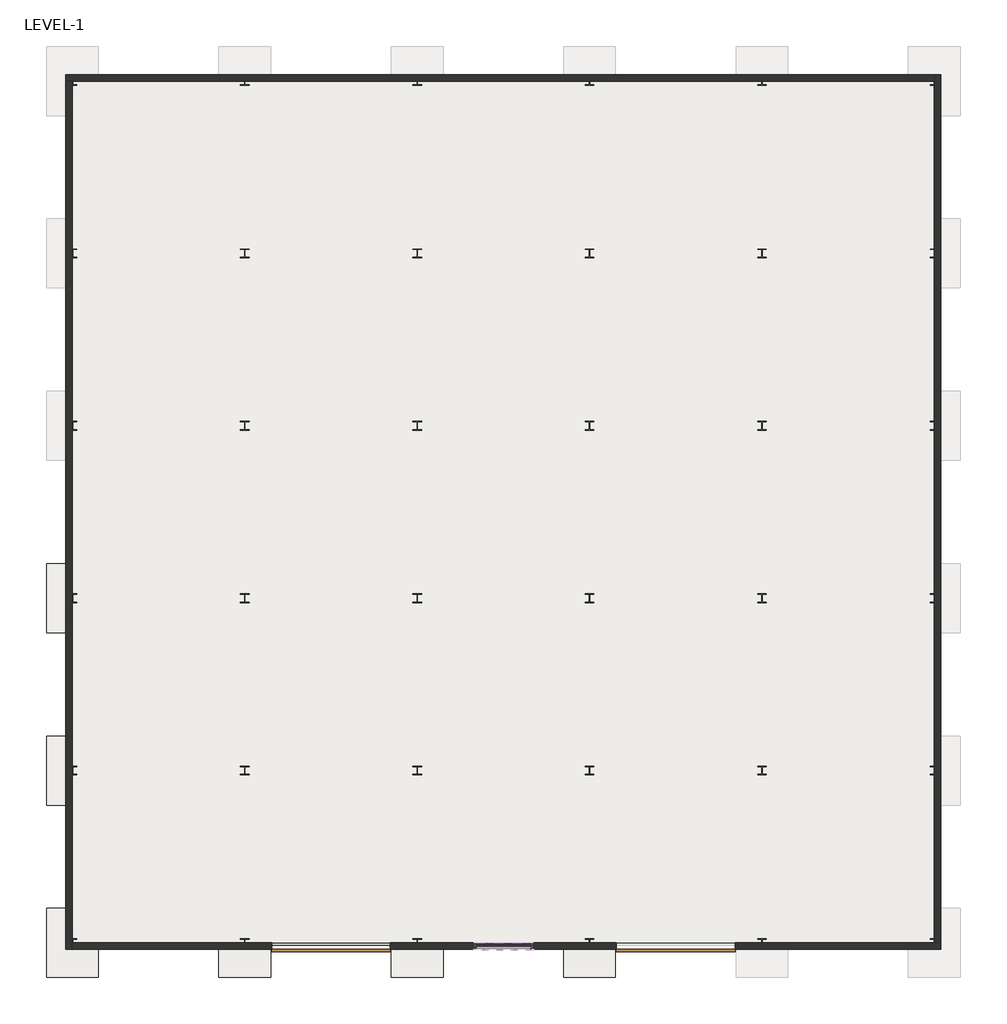
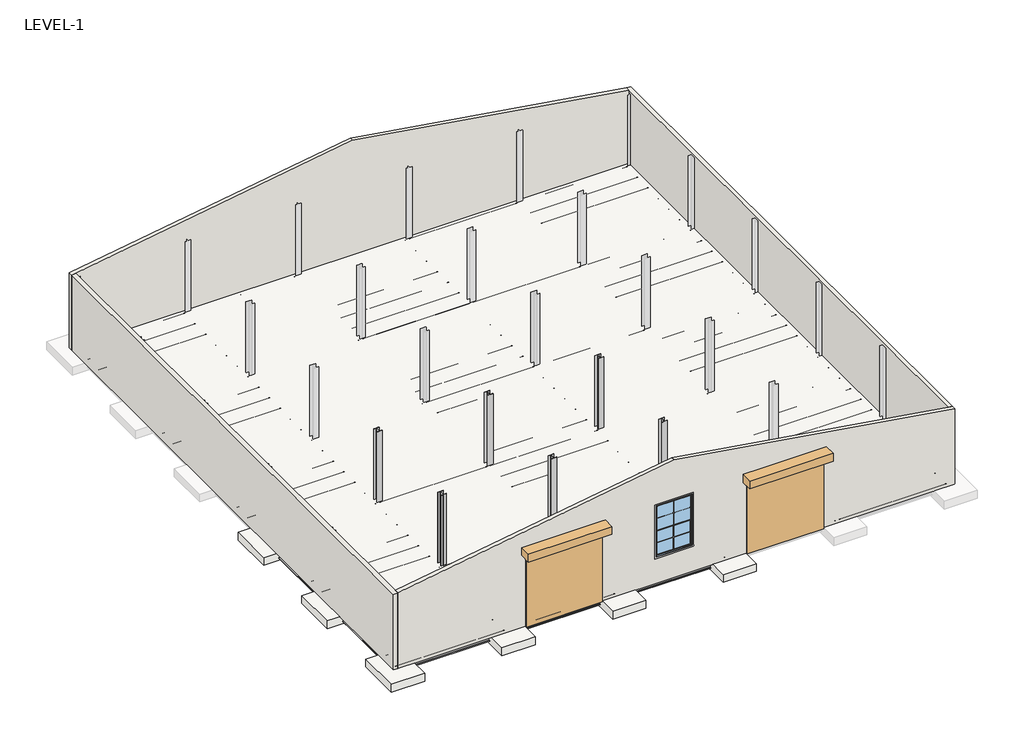
# One storey, part 1 of 3: 51 beams, 13 slabs, 12 columns, 4 walls, 2 doors, 1 window.
"""IFC4 building model written with IfcOpenShell, lengths in millimetres."""

from ifc_helpers import new_model, si_unit, frame, origin, place, context, project, spatial, polyline, outline, extrude, faceted_brep, transform, mapped, element, save
from components import ub_universal_beams_ub305x165x40_15f88fa9, ub_universal_beams_ub305x165x40_f918ae41, ub_universal_beams_ub305x165x40_f15b2736, ub_universal_beams_ub305x165x40_694d595e, uc_universal_columns_column_uc305x305x97_11a20181, m_door_overhead_rolling_4200_x_4200mm_2c196bb8, m_door_overhead_rolling_4200_x_4200mm_f21f583b, slab_7b69f09a, m_window_double_hung_2000_x_3000mm_b5dbafc5

model = new_model("IFC4")

# Units and contexts
model_context = context("Model", 3, world=origin())
ifc_project = project(units=[si_unit("LENGTHUNIT", "METRE", prefix="MILLI")], contexts=[model_context])

# Site, building, storey
site = spatial("IfcSite", under=ifc_project)
building = spatial("IfcBuilding", under=site)
storey = spatial("IfcBuildingStorey", under=building, Name="LEVEL-1", Elevation=0.0)

# Beams
placement = place(None, origin())
ub_universal_beams_ub305x165x40_shape = ub_universal_beams_ub305x165x40_15f88fa9(model_context)
element("IfcBeam", 1, ObjectType="UB-Universal Beams : UB305x165x40", at=placement, inside=storey, context=model_context, shape_type="MappedRepresentation", body=[
    mapped(ub_universal_beams_ub305x165x40_shape, transform((-15492.3332854, -104.4765895, -151.7), x_axis=(1.0, 0.0, 0.0), y_axis=(0.0, 1.0, 0.0), z_axis=(0.0, 0.0, 1.0))),
])
element("IfcBeam", 2, ObjectType="UB-Universal Beams : UB305x165x40", at=placement, inside=storey, context=model_context, shape_type="MappedRepresentation", body=[
    mapped(ub_universal_beams_ub305x165x40_shape, transform((-15492.3332854, -1120.4765895, -151.7), x_axis=(1.0, 0.0, 0.0), y_axis=(0.0, 1.0, 0.0), z_axis=(0.0, 0.0, 1.0))),
])
element("IfcBeam", 3, ObjectType="UB-Universal Beams : UB305x165x40", at=placement, inside=storey, context=model_context, shape_type="MappedRepresentation", body=[
    mapped(ub_universal_beams_ub305x165x40_shape, transform((-15492.3332854, -3152.4765895, -151.7), x_axis=(1.0, 0.0, 0.0), y_axis=(0.0, 1.0, 0.0), z_axis=(0.0, 0.0, 1.0))),
])
element("IfcBeam", 4, ObjectType="UB-Universal Beams : UB305x165x40", at=placement, inside=storey, context=model_context, shape_type="MappedRepresentation", body=[
    mapped(ub_universal_beams_ub305x165x40_shape, transform((-15492.3332854, -4168.4765895, -151.7), x_axis=(1.0, 0.0, 0.0), y_axis=(0.0, 1.0, 0.0), z_axis=(0.0, 0.0, 1.0))),
])
element("IfcBeam", 5, ObjectType="UB-Universal Beams : UB305x165x40", at=placement, inside=storey, context=model_context, shape_type="MappedRepresentation", body=[
    mapped(ub_universal_beams_ub305x165x40_shape, transform((-15492.3332854, -5184.4765895, -151.7), x_axis=(1.0, 0.0, 0.0), y_axis=(0.0, 1.0, 0.0), z_axis=(0.0, 0.0, 1.0))),
])
element("IfcBeam", 6, ObjectType="UB-Universal Beams : UB305x165x40", at=placement, inside=storey, context=model_context, shape_type="MappedRepresentation", body=[
    mapped(ub_universal_beams_ub305x165x40_shape, transform((-15492.3332854, -6200.4765895, -151.7), x_axis=(1.0, 0.0, 0.0), y_axis=(0.0, 1.0, 0.0), z_axis=(0.0, 0.0, 1.0))),
])
element("IfcBeam", 7, ObjectType="UB-Universal Beams : UB305x165x40", at=placement, inside=storey, context=model_context, shape_type="MappedRepresentation", body=[
    mapped(ub_universal_beams_ub305x165x40_shape, transform((-15492.3332854, -7216.4765895, -151.7), x_axis=(1.0, 0.0, 0.0), y_axis=(0.0, 1.0, 0.0), z_axis=(0.0, 0.0, 1.0))),
])
element("IfcBeam", 8, ObjectType="UB-Universal Beams : UB305x165x40", at=placement, inside=storey, context=model_context, shape_type="MappedRepresentation", body=[
    mapped(ub_universal_beams_ub305x165x40_shape, transform((-15492.3332854, -9248.4765895, -151.7), x_axis=(1.0, 0.0, 0.0), y_axis=(0.0, 1.0, 0.0), z_axis=(0.0, 0.0, 1.0))),
])
element("IfcBeam", 9, ObjectType="UB-Universal Beams : UB305x165x40", at=placement, inside=storey, context=model_context, shape_type="MappedRepresentation", body=[
    mapped(ub_universal_beams_ub305x165x40_shape, transform((-15492.3332854, -10264.4765895, -151.7), x_axis=(1.0, 0.0, 0.0), y_axis=(0.0, 1.0, 0.0), z_axis=(0.0, 0.0, 1.0))),
])
element("IfcBeam", 10, ObjectType="UB-Universal Beams : UB305x165x40", at=placement, inside=storey, context=model_context, shape_type="MappedRepresentation", body=[
    mapped(ub_universal_beams_ub305x165x40_shape, transform((-15492.3332854, -11280.4765895, -151.7), x_axis=(1.0, 0.0, 0.0), y_axis=(0.0, 1.0, 0.0), z_axis=(0.0, 0.0, 1.0))),
])
element("IfcBeam", 11, ObjectType="UB-Universal Beams : UB305x165x40", at=placement, inside=storey, context=model_context, shape_type="MappedRepresentation", body=[
    mapped(ub_universal_beams_ub305x165x40_shape, transform((-15492.3332854, -12296.4765895, -151.7), x_axis=(1.0, 0.0, 0.0), y_axis=(0.0, 1.0, 0.0), z_axis=(0.0, 0.0, 1.0))),
])
element("IfcBeam", 12, ObjectType="UB-Universal Beams : UB305x165x40", at=placement, inside=storey, context=model_context, shape_type="MappedRepresentation", body=[
    mapped(ub_universal_beams_ub305x165x40_shape, transform((-15492.3332854, -13312.4765895, -151.7), x_axis=(1.0, 0.0, 0.0), y_axis=(0.0, 1.0, 0.0), z_axis=(0.0, 0.0, 1.0))),
])
element("IfcBeam", 13, ObjectType="UB-Universal Beams : UB305x165x40", at=placement, inside=storey, context=model_context, shape_type="MappedRepresentation", body=[
    mapped(ub_universal_beams_ub305x165x40_shape, transform((-3300.3332854, -104.4765895, -151.7), x_axis=(1.0, 0.0, 0.0), y_axis=(0.0, 1.0, 0.0), z_axis=(0.0, 0.0, 1.0))),
])
element("IfcBeam", 14, ObjectType="UB-Universal Beams : UB305x165x40", at=placement, inside=storey, context=model_context, shape_type="MappedRepresentation", body=[
    mapped(ub_universal_beams_ub305x165x40_shape, transform((-3300.3332854, -1120.4765895, -151.7), x_axis=(1.0, 0.0, 0.0), y_axis=(0.0, 1.0, 0.0), z_axis=(0.0, 0.0, 1.0))),
])
element("IfcBeam", 15, ObjectType="UB-Universal Beams : UB305x165x40", at=placement, inside=storey, context=model_context, shape_type="MappedRepresentation", body=[
    mapped(ub_universal_beams_ub305x165x40_shape, transform((-3300.3332854, -3152.4765895, -151.7), x_axis=(1.0, 0.0, 0.0), y_axis=(0.0, 1.0, 0.0), z_axis=(0.0, 0.0, 1.0))),
])
element("IfcBeam", 16, ObjectType="UB-Universal Beams : UB305x165x40", at=placement, inside=storey, context=model_context, shape_type="MappedRepresentation", body=[
    mapped(ub_universal_beams_ub305x165x40_shape, transform((-3300.3332854, -4168.4765895, -151.7), x_axis=(1.0, 0.0, 0.0), y_axis=(0.0, 1.0, 0.0), z_axis=(0.0, 0.0, 1.0))),
])
element("IfcBeam", 17, ObjectType="UB-Universal Beams : UB305x165x40", at=placement, inside=storey, context=model_context, shape_type="MappedRepresentation", body=[
    mapped(ub_universal_beams_ub305x165x40_shape, transform((-3300.3332854, -5184.4765895, -151.7), x_axis=(1.0, 0.0, 0.0), y_axis=(0.0, 1.0, 0.0), z_axis=(0.0, 0.0, 1.0))),
])
element("IfcBeam", 18, ObjectType="UB-Universal Beams : UB305x165x40", at=placement, inside=storey, context=model_context, shape_type="MappedRepresentation", body=[
    mapped(ub_universal_beams_ub305x165x40_shape, transform((-3300.3332854, -6200.4765895, -151.7), x_axis=(1.0, 0.0, 0.0), y_axis=(0.0, 1.0, 0.0), z_axis=(0.0, 0.0, 1.0))),
])
element("IfcBeam", 19, ObjectType="UB-Universal Beams : UB305x165x40", at=placement, inside=storey, context=model_context, shape_type="MappedRepresentation", body=[
    mapped(ub_universal_beams_ub305x165x40_shape, transform((-3300.3332854, -7216.4765895, -151.7), x_axis=(1.0, 0.0, 0.0), y_axis=(0.0, 1.0, 0.0), z_axis=(0.0, 0.0, 1.0))),
])
element("IfcBeam", 20, ObjectType="UB-Universal Beams : UB305x165x40", at=placement, inside=storey, context=model_context, shape_type="MappedRepresentation", body=[
    mapped(ub_universal_beams_ub305x165x40_shape, transform((-3300.3332854, -9248.4765895, -151.7), x_axis=(1.0, 0.0, 0.0), y_axis=(0.0, 1.0, 0.0), z_axis=(0.0, 0.0, 1.0))),
])
element("IfcBeam", 21, ObjectType="UB-Universal Beams : UB305x165x40", at=placement, inside=storey, context=model_context, shape_type="MappedRepresentation", body=[
    mapped(ub_universal_beams_ub305x165x40_shape, transform((-3300.3332854, -10264.4765895, -151.7), x_axis=(1.0, 0.0, 0.0), y_axis=(0.0, 1.0, 0.0), z_axis=(0.0, 0.0, 1.0))),
])
element("IfcBeam", 22, ObjectType="UB-Universal Beams : UB305x165x40", at=placement, inside=storey, context=model_context, shape_type="MappedRepresentation", body=[
    mapped(ub_universal_beams_ub305x165x40_shape, transform((-3300.3332854, -11280.4765895, -151.7), x_axis=(1.0, 0.0, 0.0), y_axis=(0.0, 1.0, 0.0), z_axis=(0.0, 0.0, 1.0))),
])
element("IfcBeam", 23, ObjectType="UB-Universal Beams : UB305x165x40", at=placement, inside=storey, context=model_context, shape_type="MappedRepresentation", body=[
    mapped(ub_universal_beams_ub305x165x40_shape, transform((-3300.3332854, -12296.4765895, -151.7), x_axis=(1.0, 0.0, 0.0), y_axis=(0.0, 1.0, 0.0), z_axis=(0.0, 0.0, 1.0))),
])
element("IfcBeam", 24, ObjectType="UB-Universal Beams : UB305x165x40", at=placement, inside=storey, context=model_context, shape_type="MappedRepresentation", body=[
    mapped(ub_universal_beams_ub305x165x40_shape, transform((-3300.3332854, -13312.4765895, -151.7), x_axis=(1.0, 0.0, 0.0), y_axis=(0.0, 1.0, 0.0), z_axis=(0.0, 0.0, 1.0))),
])
element("IfcBeam", 25, ObjectType="UB-Universal Beams : UB305x165x40", at=placement, inside=storey, context=model_context, shape_type="MappedRepresentation", body=[
    mapped(ub_universal_beams_ub305x165x40_shape, transform((-7364.3332854, -5184.4765895, -151.7), x_axis=(0.0, -1.0, 0.0), y_axis=(1.0, 0.0, 0.0), z_axis=(0.0, 0.0, 1.0))),
])
element("IfcBeam", 26, ObjectType="UB-Universal Beams : UB305x165x40", at=placement, inside=storey, context=model_context, shape_type="MappedRepresentation", body=[
    mapped(ub_universal_beams_ub305x165x40_shape, transform((-8380.3332854, -5184.4765895, -151.7), x_axis=(0.0, -1.0, 0.0), y_axis=(1.0, 0.0, 0.0), z_axis=(0.0, 0.0, 1.0))),
])
element("IfcBeam", 27, ObjectType="UB-Universal Beams : UB305x165x40", at=placement, inside=storey, context=model_context, shape_type="MappedRepresentation", body=[
    mapped(ub_universal_beams_ub305x165x40_shape, transform((-9396.3332854, -5184.4765895, -151.7), x_axis=(0.0, -1.0, 0.0), y_axis=(1.0, 0.0, 0.0), z_axis=(0.0, 0.0, 1.0))),
])
element("IfcBeam", 28, ObjectType="UB-Universal Beams : UB305x165x40", at=placement, inside=storey, context=model_context, shape_type="MappedRepresentation", body=[
    mapped(ub_universal_beams_ub305x165x40_shape, transform((-10412.3332854, -5184.4765895, -151.7), x_axis=(0.0, -1.0, 0.0), y_axis=(1.0, 0.0, 0.0), z_axis=(0.0, 0.0, 1.0))),
])
element("IfcBeam", 29, ObjectType="UB-Universal Beams : UB305x165x40", at=placement, inside=storey, context=model_context, shape_type="MappedRepresentation", body=[
    mapped(ub_universal_beams_ub305x165x40_shape, transform((-11428.3332854, -5184.4765895, -151.7), x_axis=(0.0, -1.0, 0.0), y_axis=(1.0, 0.0, 0.0), z_axis=(0.0, 0.0, 1.0))),
])
element("IfcBeam", 30, ObjectType="UB-Universal Beams : UB305x165x40", at=placement, inside=storey, context=model_context, shape_type="MappedRepresentation", body=[
    mapped(ub_universal_beams_ub305x165x40_shape, transform((-7364.3332854, -11280.4765895, -151.7), x_axis=(0.0, -1.0, 0.0), y_axis=(1.0, 0.0, 0.0), z_axis=(0.0, 0.0, 1.0))),
])
element("IfcBeam", 31, ObjectType="UB-Universal Beams : UB305x165x40", at=placement, inside=storey, context=model_context, shape_type="MappedRepresentation", body=[
    mapped(ub_universal_beams_ub305x165x40_shape, transform((-8380.3332854, -11280.4765895, -151.7), x_axis=(0.0, -1.0, 0.0), y_axis=(1.0, 0.0, 0.0), z_axis=(0.0, 0.0, 1.0))),
])
element("IfcBeam", 32, ObjectType="UB-Universal Beams : UB305x165x40", at=placement, inside=storey, context=model_context, shape_type="MappedRepresentation", body=[
    mapped(ub_universal_beams_ub305x165x40_shape, transform((-9396.3332854, -11280.4765895, -151.7), x_axis=(0.0, -1.0, 0.0), y_axis=(1.0, 0.0, 0.0), z_axis=(0.0, 0.0, 1.0))),
])
element("IfcBeam", 33, ObjectType="UB-Universal Beams : UB305x165x40", at=placement, inside=storey, context=model_context, shape_type="MappedRepresentation", body=[
    mapped(ub_universal_beams_ub305x165x40_shape, transform((-10412.3332854, -11280.4765895, -151.7), x_axis=(0.0, -1.0, 0.0), y_axis=(1.0, 0.0, 0.0), z_axis=(0.0, 0.0, 1.0))),
])
element("IfcBeam", 34, ObjectType="UB-Universal Beams : UB305x165x40", at=placement, inside=storey, context=model_context, shape_type="MappedRepresentation", body=[
    mapped(ub_universal_beams_ub305x165x40_shape, transform((-11428.3332854, -11280.4765895, -151.7), x_axis=(0.0, -1.0, 0.0), y_axis=(1.0, 0.0, 0.0), z_axis=(0.0, 0.0, 1.0))),
])
element("IfcBeam", 35, ObjectType="UB-Universal Beams : UB305x165x40", at=placement, inside=storey, context=model_context, shape_type="MappedRepresentation", body=[
    mapped(ub_universal_beams_ub305x165x40_shape, transform((-9396.3332854, -14328.4765895, -151.7), x_axis=(1.0, 0.0, 0.0), y_axis=(0.0, 1.0, 0.0), z_axis=(0.0, 0.0, 1.0))),
])
element("IfcBeam", 36, ObjectType="UB-Universal Beams : UB305x165x40", at=placement, inside=storey, context=model_context, shape_type="MappedRepresentation", body=[
    mapped(ub_universal_beams_ub305x165x40_shape, transform((-3300.3332854, -14328.4765895, -151.7), x_axis=(1.0, 0.0, 0.0), y_axis=(0.0, 1.0, 0.0), z_axis=(0.0, 0.0, 1.0))),
])
element("IfcBeam", 37, ObjectType="UB-Universal Beams : UB305x165x40", at=placement, inside=storey, context=model_context, shape_type="MappedRepresentation", body=[
    mapped(ub_universal_beams_ub305x165x40_shape, transform((-9396.3332854, -8232.4765895, -151.7), x_axis=(1.0, 0.0, 0.0), y_axis=(0.0, 1.0, 0.0), z_axis=(0.0, 0.0, 1.0))),
])
element("IfcBeam", 38, ObjectType="UB-Universal Beams : UB305x165x40", at=placement, inside=storey, context=model_context, shape_type="MappedRepresentation", body=[
    mapped(ub_universal_beams_ub305x165x40_shape, transform((-3300.3332854, -8232.4765895, -151.7), x_axis=(1.0, 0.0, 0.0), y_axis=(0.0, 1.0, 0.0), z_axis=(0.0, 0.0, 1.0))),
])
element("IfcBeam", 39, ObjectType="UB-Universal Beams : UB305x165x40", at=placement, inside=storey, context=model_context, shape_type="MappedRepresentation", body=[
    mapped(ub_universal_beams_ub305x165x40_shape, transform((-9396.3332854, -2136.4765895, -151.7), x_axis=(1.0, 0.0, 0.0), y_axis=(0.0, 1.0, 0.0), z_axis=(0.0, 0.0, 1.0))),
])
element("IfcBeam", 40, ObjectType="UB-Universal Beams : UB305x165x40", at=placement, inside=storey, context=model_context, shape_type="MappedRepresentation", body=[
    mapped(ub_universal_beams_ub305x165x40_shape, transform((-3300.3332854, -2136.4765895, -151.7), x_axis=(1.0, 0.0, 0.0), y_axis=(0.0, 1.0, 0.0), z_axis=(0.0, 0.0, 1.0))),
])
element("IfcBeam", 41, ObjectType="UB-Universal Beams : UB305x165x40", at=placement, inside=storey, context=model_context, shape_type="MappedRepresentation", body=[
    mapped(ub_universal_beams_ub305x165x40_shape, transform((-18540.3332854, -5184.4765895, -151.7), x_axis=(0.0, 1.0, 0.0), y_axis=(-1.0, 0.0, 0.0), z_axis=(0.0, 0.0, 1.0))),
])
ub_universal_beams_ub305x165x40_2_shape = ub_universal_beams_ub305x165x40_f918ae41(model_context)
element("IfcBeam", 42, ObjectType="UB-Universal Beams : UB305x165x40", at=placement, inside=storey, context=model_context, shape_type="MappedRepresentation", body=[
    mapped(ub_universal_beams_ub305x165x40_2_shape, transform((-252.3332854, -5184.4765895, -151.7), x_axis=(0.0, 1.0, 0.0), y_axis=(-1.0, 0.0, 0.0), z_axis=(0.0, 0.0, 1.0))),
])
element("IfcBeam", 43, ObjectType="UB-Universal Beams : UB305x165x40", at=placement, inside=storey, context=model_context, shape_type="MappedRepresentation", body=[
    mapped(ub_universal_beams_ub305x165x40_2_shape, transform((-6348.3332854, -5184.4765895, -151.7), x_axis=(0.0, 1.0, 0.0), y_axis=(-1.0, 0.0, 0.0), z_axis=(0.0, 0.0, 1.0))),
])
element("IfcBeam", 44, ObjectType="UB-Universal Beams : UB305x165x40", at=placement, inside=storey, context=model_context, shape_type="MappedRepresentation", body=[
    mapped(ub_universal_beams_ub305x165x40_2_shape, transform((-12444.3332854, -5184.4765895, -151.7), x_axis=(0.0, 1.0, 0.0), y_axis=(-1.0, 0.0, 0.0), z_axis=(0.0, 0.0, 1.0))),
])
ub_universal_beams_ub305x165x40_3_shape = ub_universal_beams_ub305x165x40_f15b2736(model_context)
element("IfcBeam", 45, ObjectType="UB-Universal Beams : UB305x165x40", at=placement, inside=storey, context=model_context, shape_type="MappedRepresentation", body=[
    mapped(ub_universal_beams_ub305x165x40_3_shape, transform((-15549.3308854, -14328.4765895, -151.7), x_axis=(1.0, 0.0, 0.0), y_axis=(0.0, 1.0, 0.0), z_axis=(0.0, 0.0, 1.0))),
])
element("IfcBeam", 46, ObjectType="UB-Universal Beams : UB305x165x40", at=placement, inside=storey, context=model_context, shape_type="MappedRepresentation", body=[
    mapped(ub_universal_beams_ub305x165x40_3_shape, transform((-15549.3308854, -8232.4765895, -151.7), x_axis=(1.0, 0.0, 0.0), y_axis=(0.0, 1.0, 0.0), z_axis=(0.0, 0.0, 1.0))),
])
element("IfcBeam", 47, ObjectType="UB-Universal Beams : UB305x165x40", at=placement, inside=storey, context=model_context, shape_type="MappedRepresentation", body=[
    mapped(ub_universal_beams_ub305x165x40_3_shape, transform((-15549.3308854, -2136.4765895, -151.7), x_axis=(1.0, 0.0, 0.0), y_axis=(0.0, 1.0, 0.0), z_axis=(0.0, 0.0, 1.0))),
])
ub_universal_beams_ub305x165x40_4_shape = ub_universal_beams_ub305x165x40_694d595e(model_context)
element("IfcBeam", 48, ObjectType="UB-Universal Beams : UB305x165x40", at=placement, inside=storey, context=model_context, shape_type="MappedRepresentation", body=[
    mapped(ub_universal_beams_ub305x165x40_4_shape, transform((-252.3332854, -11337.6265895, -151.7), x_axis=(0.0, 1.0, 0.0), y_axis=(-1.0, 0.0, 0.0), z_axis=(0.0, 0.0, 1.0))),
])
element("IfcBeam", 49, ObjectType="UB-Universal Beams : UB305x165x40", at=placement, inside=storey, context=model_context, shape_type="MappedRepresentation", body=[
    mapped(ub_universal_beams_ub305x165x40_4_shape, transform((-6348.3332854, -11337.6265895, -151.7), x_axis=(0.0, 1.0, 0.0), y_axis=(-1.0, 0.0, 0.0), z_axis=(0.0, 0.0, 1.0))),
])
element("IfcBeam", 50, ObjectType="UB-Universal Beams : UB305x165x40", at=placement, inside=storey, context=model_context, shape_type="MappedRepresentation", body=[
    mapped(ub_universal_beams_ub305x165x40_4_shape, transform((-12444.3332854, -11337.6265895, -151.7), x_axis=(0.0, 1.0, 0.0), y_axis=(-1.0, 0.0, 0.0), z_axis=(0.0, 0.0, 1.0))),
])
element("IfcBeam", 51, ObjectType="UB-Universal Beams : UB305x165x40", at=placement, inside=storey, context=model_context, shape_type="MappedRepresentation", body=[
    mapped(ub_universal_beams_ub305x165x40_4_shape, transform((-18540.3332854, -11337.6265895, -151.7), x_axis=(0.0, 1.0, 0.0), y_axis=(-1.0, 0.0, 0.0), z_axis=(0.0, 0.0, 1.0))),
])

# Columns
uc_universal_columns_column_uc305x305x97_shape = uc_universal_columns_column_uc305x305x97_11a20181(model_context)
element("IfcColumn", 52, ObjectType="UC-Universal Columns-Column : UC305x305x97", at=placement, inside=storey, context=model_context, shape_type="MappedRepresentation", body=[
    mapped(uc_universal_columns_column_uc305x305x97_shape, transform((-252.3332854, -14328.4765895, 0.0), x_axis=(1.0, 0.0, 0.0), y_axis=(0.0, 1.0, 0.0), z_axis=(0.0, 0.0, 1.0))),
])
element("IfcColumn", 53, ObjectType="UC-Universal Columns-Column : UC305x305x97", at=placement, inside=storey, context=model_context, shape_type="MappedRepresentation", body=[
    mapped(uc_universal_columns_column_uc305x305x97_shape, transform((-6348.3332854, -14328.4765895, 0.0), x_axis=(1.0, 0.0, 0.0), y_axis=(0.0, 1.0, 0.0), z_axis=(0.0, 0.0, 1.0))),
])
element("IfcColumn", 54, ObjectType="UC-Universal Columns-Column : UC305x305x97", at=placement, inside=storey, context=model_context, shape_type="MappedRepresentation", body=[
    mapped(uc_universal_columns_column_uc305x305x97_shape, transform((-12444.3332854, -14328.4765895, 0.0), x_axis=(1.0, 0.0, 0.0), y_axis=(0.0, 1.0, 0.0), z_axis=(0.0, 0.0, 1.0))),
])
element("IfcColumn", 55, ObjectType="UC-Universal Columns-Column : UC305x305x97", at=placement, inside=storey, context=model_context, shape_type="MappedRepresentation", body=[
    mapped(uc_universal_columns_column_uc305x305x97_shape, transform((-18540.3332854, -14328.4765895, 0.0), x_axis=(1.0, 0.0, 0.0), y_axis=(0.0, 1.0, 0.0), z_axis=(0.0, 0.0, 1.0))),
])
element("IfcColumn", 56, ObjectType="UC-Universal Columns-Column : UC305x305x97", at=placement, inside=storey, context=model_context, shape_type="MappedRepresentation", body=[
    mapped(uc_universal_columns_column_uc305x305x97_shape, transform((-252.3332854, -8232.4765895, 0.0), x_axis=(1.0, 0.0, 0.0), y_axis=(0.0, 1.0, 0.0), z_axis=(0.0, 0.0, 1.0))),
])
element("IfcColumn", 57, ObjectType="UC-Universal Columns-Column : UC305x305x97", at=placement, inside=storey, context=model_context, shape_type="MappedRepresentation", body=[
    mapped(uc_universal_columns_column_uc305x305x97_shape, transform((-6348.3332854, -8232.4765895, 0.0), x_axis=(1.0, 0.0, 0.0), y_axis=(0.0, 1.0, 0.0), z_axis=(0.0, 0.0, 1.0))),
])
element("IfcColumn", 58, ObjectType="UC-Universal Columns-Column : UC305x305x97", at=placement, inside=storey, context=model_context, shape_type="MappedRepresentation", body=[
    mapped(uc_universal_columns_column_uc305x305x97_shape, transform((-12444.3332854, -8232.4765895, 0.0), x_axis=(1.0, 0.0, 0.0), y_axis=(0.0, 1.0, 0.0), z_axis=(0.0, 0.0, 1.0))),
])
element("IfcColumn", 59, ObjectType="UC-Universal Columns-Column : UC305x305x97", at=placement, inside=storey, context=model_context, shape_type="MappedRepresentation", body=[
    mapped(uc_universal_columns_column_uc305x305x97_shape, transform((-18540.3332854, -8232.4765895, 0.0), x_axis=(1.0, 0.0, 0.0), y_axis=(0.0, 1.0, 0.0), z_axis=(0.0, 0.0, 1.0))),
])
element("IfcColumn", 60, ObjectType="UC-Universal Columns-Column : UC305x305x97", at=placement, inside=storey, context=model_context, shape_type="MappedRepresentation", body=[
    mapped(uc_universal_columns_column_uc305x305x97_shape, transform((-252.3332854, -2136.4765895, 0.0), x_axis=(1.0, 0.0, 0.0), y_axis=(0.0, 1.0, 0.0), z_axis=(0.0, 0.0, 1.0))),
])
element("IfcColumn", 61, ObjectType="UC-Universal Columns-Column : UC305x305x97", at=placement, inside=storey, context=model_context, shape_type="MappedRepresentation", body=[
    mapped(uc_universal_columns_column_uc305x305x97_shape, transform((-6348.3332854, -2136.4765895, 0.0), x_axis=(1.0, 0.0, 0.0), y_axis=(0.0, 1.0, 0.0), z_axis=(0.0, 0.0, 1.0))),
])
element("IfcColumn", 62, ObjectType="UC-Universal Columns-Column : UC305x305x97", at=placement, inside=storey, context=model_context, shape_type="MappedRepresentation", body=[
    mapped(uc_universal_columns_column_uc305x305x97_shape, transform((-12444.3332854, -2136.4765895, 0.0), x_axis=(1.0, 0.0, 0.0), y_axis=(0.0, 1.0, 0.0), z_axis=(0.0, 0.0, 1.0))),
])
element("IfcColumn", 63, ObjectType="UC-Universal Columns-Column : UC305x305x97", at=placement, inside=storey, context=model_context, shape_type="MappedRepresentation", body=[
    mapped(uc_universal_columns_column_uc305x305x97_shape, transform((-18540.3332854, -2136.4765895, 0.0), x_axis=(1.0, 0.0, 0.0), y_axis=(0.0, 1.0, 0.0), z_axis=(0.0, 0.0, 1.0))),
])

# Doors
m_door_overhead_rolling_4200_x_4200mm_shape = m_door_overhead_rolling_4200_x_4200mm_2c196bb8(model_context)
element("IfcDoor", 64, ObjectType="M_Door-Overhead-Rolling : 4200 x 4200mm", at=placement, inside=storey, context=model_context, shape_type="MappedRepresentation", body=[
    mapped(m_door_overhead_rolling_4200_x_4200mm_shape, transform((-9396.3332854, -14442.7765895, 0.0), x_axis=(1.0, 0.0, 0.0), y_axis=(0.0, 1.0, 0.0), z_axis=(0.0, 0.0, 1.0))),
])
m_door_overhead_rolling_4200_x_4200mm_2_shape = m_door_overhead_rolling_4200_x_4200mm_f21f583b(model_context)
element("IfcDoor", 65, ObjectType="M_Door-Overhead-Rolling : 4200 x 4200mm", at=placement, inside=storey, context=model_context, shape_type="MappedRepresentation", body=[
    mapped(m_door_overhead_rolling_4200_x_4200mm_2_shape, transform((2795.6667146, -14442.7765895, 0.0), x_axis=(-1.0, 0.0, 0.0), y_axis=(0.0, -1.0, 0.0), z_axis=(0.0, 0.0, 1.0))),
])

# Slabs
slab_shape = slab_7b69f09a(model_context)
element("IfcSlab", 66, ObjectType="Footing-Rectangular : 96\" x 72\" x 18\"", at=placement, inside=storey, context=model_context, shape_type="MappedRepresentation", body=[
    mapped(slab_shape, transform((-252.3332854, -14328.4765895, 0.0), x_axis=(1.0, 0.0, 0.0), y_axis=(0.0, 1.0, 0.0), z_axis=(0.0, 0.0, 1.0))),
])
element("IfcSlab", 67, ObjectType="Footing-Rectangular : 96\" x 72\" x 18\"", at=placement, inside=storey, context=model_context, shape_type="MappedRepresentation", body=[
    mapped(slab_shape, transform((-6348.3332854, -14328.4765895, 0.0), x_axis=(1.0, 0.0, 0.0), y_axis=(0.0, 1.0, 0.0), z_axis=(0.0, 0.0, 1.0))),
])
element("IfcSlab", 68, ObjectType="Footing-Rectangular : 96\" x 72\" x 18\"", at=placement, inside=storey, context=model_context, shape_type="MappedRepresentation", body=[
    mapped(slab_shape, transform((-12444.3332854, -14328.4765895, 0.0), x_axis=(1.0, 0.0, 0.0), y_axis=(0.0, 1.0, 0.0), z_axis=(0.0, 0.0, 1.0))),
])
element("IfcSlab", 69, ObjectType="Footing-Rectangular : 96\" x 72\" x 18\"", at=placement, inside=storey, context=model_context, shape_type="MappedRepresentation", body=[
    mapped(slab_shape, transform((-18540.3332854, -14328.4765895, 0.0), x_axis=(1.0, 0.0, 0.0), y_axis=(0.0, 1.0, 0.0), z_axis=(0.0, 0.0, 1.0))),
])
element("IfcSlab", 70, ObjectType="Footing-Rectangular : 96\" x 72\" x 18\"", at=placement, inside=storey, context=model_context, shape_type="MappedRepresentation", body=[
    mapped(slab_shape, transform((-252.3332854, -8232.4765895, 0.0), x_axis=(1.0, 0.0, 0.0), y_axis=(0.0, 1.0, 0.0), z_axis=(0.0, 0.0, 1.0))),
])
element("IfcSlab", 71, ObjectType="Footing-Rectangular : 96\" x 72\" x 18\"", at=placement, inside=storey, context=model_context, shape_type="MappedRepresentation", body=[
    mapped(slab_shape, transform((-6348.3332854, -8232.4765895, 0.0), x_axis=(1.0, 0.0, 0.0), y_axis=(0.0, 1.0, 0.0), z_axis=(0.0, 0.0, 1.0))),
])
element("IfcSlab", 72, ObjectType="Footing-Rectangular : 96\" x 72\" x 18\"", at=placement, inside=storey, context=model_context, shape_type="MappedRepresentation", body=[
    mapped(slab_shape, transform((-12444.3332854, -8232.4765895, 0.0), x_axis=(1.0, 0.0, 0.0), y_axis=(0.0, 1.0, 0.0), z_axis=(0.0, 0.0, 1.0))),
])
element("IfcSlab", 73, ObjectType="Footing-Rectangular : 96\" x 72\" x 18\"", at=placement, inside=storey, context=model_context, shape_type="MappedRepresentation", body=[
    mapped(slab_shape, transform((-18540.3332854, -8232.4765895, 0.0), x_axis=(1.0, 0.0, 0.0), y_axis=(0.0, 1.0, 0.0), z_axis=(0.0, 0.0, 1.0))),
])
element("IfcSlab", 74, ObjectType="Footing-Rectangular : 96\" x 72\" x 18\"", at=placement, inside=storey, context=model_context, shape_type="MappedRepresentation", body=[
    mapped(slab_shape, transform((-252.3332854, -2136.4765895, 0.0), x_axis=(1.0, 0.0, 0.0), y_axis=(0.0, 1.0, 0.0), z_axis=(0.0, 0.0, 1.0))),
])
element("IfcSlab", 75, ObjectType="Footing-Rectangular : 96\" x 72\" x 18\"", at=placement, inside=storey, context=model_context, shape_type="MappedRepresentation", body=[
    mapped(slab_shape, transform((-6348.3332854, -2136.4765895, 0.0), x_axis=(1.0, 0.0, 0.0), y_axis=(0.0, 1.0, 0.0), z_axis=(0.0, 0.0, 1.0))),
])
element("IfcSlab", 76, ObjectType="Footing-Rectangular : 96\" x 72\" x 18\"", at=placement, inside=storey, context=model_context, shape_type="MappedRepresentation", body=[
    mapped(slab_shape, transform((-12444.3332854, -2136.4765895, 0.0), x_axis=(1.0, 0.0, 0.0), y_axis=(0.0, 1.0, 0.0), z_axis=(0.0, 0.0, 1.0))),
])
element("IfcSlab", 77, ObjectType="Footing-Rectangular : 96\" x 72\" x 18\"", at=placement, inside=storey, context=model_context, shape_type="MappedRepresentation", body=[
    mapped(slab_shape, transform((-18540.3332854, -2136.4765895, 0.0), x_axis=(1.0, 0.0, 0.0), y_axis=(0.0, 1.0, 0.0), z_axis=(0.0, 0.0, 1.0))),
])
element("IfcSlab", 78, ObjectType="Generic 150mm", at=placement, inside=storey, context=model_context, shape_type="SweptSolid", body=[
    extrude(outline(polyline([(11939.6667146, 16156.1968272), (11939.6667146, -14323.8031728), (-18540.3332854, -14323.8031728), (-18540.3332854, 16156.1968272), (11939.6667146, 16156.1968272)])), frame((0.0, 0.0, 0.0635964), z_axis=(0.0, 0.0, 1.0), x_axis=(1.0, 0.0, 0.0)), (0.0, 0.0, 1.0), 152.4),
])

# Walls
element("IfcWall", 79, ObjectType="Generic - 200mm", at=placement, inside=storey, context=model_context, shape_type="Brep", body=[
    faceted_brep([(-18768.6284854, 16151.5234105, 0.0), (-18540.0284854, 16151.5234105, 0.0), (11939.9715146, 16151.5234105, 0.0), (11939.9715146, 16151.5234105, 4422.0011623), (-3295.6355591, 16151.5234105, 6821.3093629), (-18540.0284854, 16151.5234105, 4420.6175634), (-18768.6284854, 16151.5234105, 4384.6175634), (-18768.6284854, 16380.1234105, 0.0), (-18768.6284854, 16380.1234105, 4384.6175634), (-3295.6355591, 16380.1234105, 6821.3093629), (11939.9715146, 16380.1234105, 4422.0011623), (11939.9715146, 16380.1234105, 0.0)], [[[0, 1, 2, 3, 4, 5, 6]], [[7, 8, 9, 10, 11]], [[2, 1, 0, 7, 11]], [[0, 6, 8, 7]], [[3, 2, 11, 10]], [[6, 5, 4, 9, 8]], [[4, 3, 10, 9]]]),
])
element("IfcWall", 80, ObjectType="Generic - 200mm", at=placement, inside=storey, context=model_context, shape_type="Brep", body=[
    faceted_brep([(-18540.0284854, -14557.0765895, 0.0), (-18540.0284854, -14328.4765895, 0.0), (-18540.0284854, 16151.5234105, 0.0), (-18540.0284854, 16151.5234105, 4420.6175634), (-18540.0284854, -14328.4765895, 4420.6175634), (-18540.0284854, -14557.0765895, 4420.6175634), (-18768.6284854, -14557.0765895, 0.0), (-18768.6284854, -14557.0765895, 4384.6175634), (-18768.6284854, 16151.5234105, 4384.6175634), (-18768.6284854, 16151.5234105, 0.0)], [[[0, 1, 2, 3, 4, 5]], [[6, 7, 8, 9]], [[2, 1, 0, 6, 9]], [[0, 5, 7, 6]], [[3, 2, 9, 8]], [[5, 4, 3, 8, 7]]]),
])
element("IfcWall", 81, ObjectType="Generic - 200mm", at=placement, inside=storey, context=model_context, shape_type="Brep", body=[
    faceted_brep([(12168.5715146, -14328.4765895, 4386.0011623), (12168.5715146, -14328.4765895, 0.0), (11939.9715146, -14328.4765895, 0.0), (4895.6667146, -14328.4765895, 0.0), (4895.6667146, -14328.4765895, 4200.0), (695.6667146, -14328.4765895, 4200.0), (695.6667146, -14328.4765895, 0.0), (-7296.3332854, -14328.4765895, 0.0), (-7296.3332854, -14328.4765895, 4200.0), (-11496.3332854, -14328.4765895, 4200.0), (-11496.3332854, -14328.4765895, 0.0), (-18540.0284854, -14328.4765895, 0.0), (-18540.0284854, -14328.4765895, 4420.6175634), (-3295.6355591, -14328.4765895, 6821.3093629), (11939.9715146, -14328.4765895, 4422.0011623), (-2300.3332854, -14328.4765895, 4512.8840152), (-4300.3332854, -14328.4765895, 4512.8840152), (-4300.3332854, -14328.4765895, 1512.8840152), (-2300.3332854, -14328.4765895, 1512.8840152), (12168.5715146, -14557.0765895, 0.0), (12168.5715146, -14557.0765895, 4386.0011623), (-3295.6355591, -14557.0765895, 6821.3093629), (-18540.0284854, -14557.0765895, 4420.6175634), (-18540.0284854, -14557.0765895, 0.0), (-11496.3332854, -14557.0765895, 0.0), (-11496.3332854, -14557.0765895, 4200.0), (-7296.3332854, -14557.0765895, 4200.0), (-7296.3332854, -14557.0765895, 0.0), (695.6667146, -14557.0765895, 0.0), (695.6667146, -14557.0765895, 4200.0), (4895.6667146, -14557.0765895, 4200.0), (4895.6667146, -14557.0765895, 0.0), (-2300.3332854, -14557.0765895, 4512.8840152), (-2300.3332854, -14557.0765895, 1512.8840152), (-4300.3332854, -14557.0765895, 1512.8840152), (-4300.3332854, -14557.0765895, 4512.8840152)], [[[0, 1, 2, 3, 4, 5, 6, 7, 8, 9, 10, 11, 12, 13, 14], [15, 16, 17, 18]], [[19, 20, 21, 22, 23, 24, 25, 26, 27, 28, 29, 30, 31], [32, 33, 34, 35]], [[1, 19, 31, 3, 2]], [[23, 11, 10, 24]], [[27, 7, 6, 28]], [[1, 0, 20, 19]], [[12, 11, 23, 22]], [[20, 0, 14, 13, 21]], [[12, 22, 21, 13]], [[26, 8, 7, 27]], [[8, 26, 25, 9]], [[9, 25, 24, 10]], [[5, 29, 28, 6]], [[29, 5, 4, 30]], [[30, 4, 3, 31]], [[33, 32, 15, 18]], [[34, 33, 18, 17]], [[35, 34, 17, 16]], [[32, 35, 16, 15]]]),
])
element("IfcWall", 82, ObjectType="Generic - 200mm", at=placement, inside=storey, context=model_context, shape_type="Brep", body=[
    faceted_brep([(11939.9715146, 16380.1234105, 0.0), (11939.9715146, 16151.5234105, 0.0), (11939.9715146, -14328.4765895, 0.0), (11939.9715146, -14328.4765895, 4422.0011623), (11939.9715146, 16151.5234105, 4422.0011623), (11939.9715146, 16380.1234105, 4422.0011623), (12168.5715146, 16380.1234105, 0.0), (12168.5715146, 16380.1234105, 4386.0011623), (12168.5715146, -14328.4765895, 4386.0011623), (12168.5715146, -14328.4765895, 0.0)], [[[0, 1, 2, 3, 4, 5]], [[6, 7, 8, 9]], [[2, 1, 0, 6, 9]], [[0, 5, 7, 6]], [[3, 2, 9, 8]], [[5, 4, 3, 8, 7]]]),
])

# Window
m_window_double_hung_2000_x_3000mm_shape = m_window_double_hung_2000_x_3000mm_b5dbafc5(model_context)
element("IfcWindow", 83, ObjectType="M_Window-Double-Hung : 2000 x 3000mm", at=placement, inside=storey, context=model_context, shape_type="MappedRepresentation", body=[
    mapped(m_window_double_hung_2000_x_3000mm_shape, transform((-3300.3332854, -14442.7765895, 598.4840152), x_axis=(-1.0, 0.0, 0.0), y_axis=(0.0, -1.0, 0.0), z_axis=(0.0, 0.0, 1.0))),
])

save(model, "model.ifc")

# Revit data of these elements
# Grids (mm)
#   "5": line (16006.314, 10055.523) -> (-22466.348, 10055.523)
#   "6": line (16006.314, 16151.523) -> (-22466.348, 16151.523)
#   "A": line (11939.667, 20647.348) -> (11939.667, -18355.996)
#   "B": line (5843.667, 20647.348) -> (5843.667, -18355.996)
#   "C": line (-252.333, 20647.348) -> (-252.333, -18355.996)
#   "D": line (-6348.333, 20647.348) -> (-6348.333, -18355.996)
#   "E": line (-12444.333, 20647.348) -> (-12444.333, -18355.996)
#   "F": line (-18540.333, 20647.348) -> (-18540.333, -18355.996)
#   "1": line (16006.314, -14328.477) -> (-22466.348, -14328.477)
#   "2": line (16006.314, -8232.477) -> (-22466.348, -8232.477)
#   "3": line (16006.314, -2136.477) -> (-22466.348, -2136.477)
#   "4": line (16006.314, 3959.523) -> (-22466.348, 3959.523)
# Type "UB-Universal Beams : UB305x165x40"
#   Section Name Key = "UB305X165X40"
#   Width = 16.5 cm
#   Web Thickness = 0.6 cm
#   Web Fillet = 0.89 cm
#   Warping Constant = 164000.0 cm⁶
#   Torsional Moment of Inertia = 14.70 cm⁴
#   Section Area = 51.3 cm²
#   Plastic Modulus weak axis = 142.0 cm³
#   Plastic Modulus strong axis = 623.0 cm³
#   Nominal Weight = 40.2999 kgf/m
#   Moment of Inertia weak axis = 764.00 cm⁴
#   Moment of Inertia strong axis = 8503.00 cm⁴
#   Height = 30.34 cm
#   Flange Thickness = 1.02 cm
#   Elastic Modulus weak axis = 92.6 cm³
#   Elastic Modulus strong axis = 560.0 cm³
#   Centroid Vertical = 15.17 cm
#   Centroid Horizontal = 8.25 cm
#   Bolt Spacing = 9.0 cm
#   Length [instance default] = 1500 mm
#   Structural Material [instance default] = Metal - Steel 43-275
#   Type Comments = ""
#   Assembly Code = ""
# Type "UC-Universal Columns-Column : UC305x305x97"
#   Section Name Key = "UC305x305x97"
#   Width = 30.53 cm
#   Web Thickness = 0.99 cm
#   Web Fillet = 1.52 cm
#   Warping Constant = 1560000.0 cm⁶
#   Torsional Moment of Inertia = 91.20 cm⁴
#   Section Area = 123.0 cm²
#   Plastic Modulus weak axis = 726.0 cm³
#   Plastic Modulus strong axis = 1592.0 cm³
#   Nominal Weight = 96.8996 kgf/m
#   Moment of Inertia weak axis = 7308.00 cm⁴
#   Moment of Inertia strong axis = 22249.00 cm⁴
#   Height = 30.79 cm
#   Flange Thickness = 1.54 cm
#   Elastic Modulus weak axis = 479.0 cm³
#   Elastic Modulus strong axis = 1445.0 cm³
#   Centroid Vertical = 15.395 cm
#   Centroid Horizontal = 15.265 cm
#   Bolt Spacing = 14.0 cm
#   Structural Material [instance default] = Metal - Steel 43-275
#   Type Comments = ""
#   Assembly Code = ""
# Type "M_Door-Overhead-Rolling : 4200 x 4200mm"
#   Type Mark = "40"
#   Construction Type Id = "MDOOR"
#   Assembly Code = "B2030400"
#   Analytic Construction = "Metal"
#   Thickness = 80 mm
#   Rough Width [instance default] = 4200 mm
#   Rough Height [instance default] = 4200 mm
#   Heat Transfer Coefficient (U) = 3.7021 W/(m²·K)
#   Height [instance default] = 4200 mm
#   Width [instance default] = 4200 mm
#   Define Thermal Properties by = 1
#   Function = 1
#   Roller Material = Steel, Paint Finish, Ivory, Matte
#   Roller Box Material = Steel, Paint Finish, Ivory, Matte
#   Visual Light Transmittance = 0
#   Solar Heat Gain Coefficient = 0
#   Wall Closure = (empty or 0)
# Type "Footing-Rectangular : 96\" x 72\" x 18\""
#   Assembly Code = "A1010100"
#   Width = 1828.8 mm
#   Length = 2438.4 mm
#   Foundation Thickness = 457.2 mm
#   Structural Material [instance default] = Concrete, Cast-in-Place gray
# Type "Generic 150mm"
#   Function = 0
#   Layers, outside or top first: 152.4 mm no material (function 1)
# Type "Generic - 200mm"
#   Layers, outside or top first: 228.6 mm no material (function 1)
# Type "M_Window-Double-Hung : 2000 x 3000mm"
#   Type Mark = "21"
#   Fire Rating = "0.5h"
#   Construction Type Id = "DG-DR"
#   Assembly Code = "B2020100"
#   Analytic Construction = "Double glazing - domestic"
#   Wall Thickness [instance default] = 150 mm
#   Window Inset [instance default] = 0 mm
#   Visual Light Transmittance = 0.81
#   Thermal Resistance (R) = 0.319569 (m²·K)/W
#   Solar Heat Gain Coefficient = 0.76
#   Muntin Width = 1847.6 mm
#   Muntin Height = 1401.575 mm
#   Interior Wall Closure [instance default] = 35.7 mm
#   Rough Width = 2015 mm
#   Rough Height = 3015 mm
#   Frame Extension [instance default] = 31.75 mm
#   Exterior Wall Closure [instance default] = 12.7 mm
#   Extension Jamb [instance default] = 35.7 mm
#   Heat Transfer Coefficient (U) = 3.12929 W/(m²·K)
#   Height = 3000 mm
#   Width = 2000 mm
#   Define Thermal Properties by = 1
#   Top Muntin Visibility = yes
#   Indicator Visibility [instance default] = yes
#   Extension Jamb Visibility [instance default] = yes
#   Interior Trim Visibility [instance default] = yes
#   Exterior Trim Visibility [instance default] = yes
#   Define Thermal Properties by = 1
#   Bottom Muntin Visibility = yes
#   Muntin Pattern = M_Muntin Pattern_2x2 : M_Muntin Pattern_2x2
#   Interior Trim Material = Wood - Stained
#   Interior Trim = M_Trim-Window-Interior-Flat : Picture Frame
#   Exterior Trim Material = Clad - White
#   Exterior Trim = M_Trim-Window-Exterior-Flat : with Sill
#   Glass Panel Material = Glass
#   Exterior Frame Material = Clad - White
#   Interior Frame Material = Wood - Stained
#   Wall Closure = (empty or 0)
# Elements 1, 2, 3, 4, 5, 6, 7, 8, 9, 10, 11, 12, 13, 14, 15, 16, 17, 18, 19, 20, 21, 22, 23, 24, 25, 26, 27, 28, 29, 30, 31, 32, 33, 34, 35, 36, 37, 38, 39, 40, 41, 42, 43, 44, 45, 46, 47, 48, 49, 50, 51 (IfcBeam, "UB-Universal Beams : UB305x165x40")
#   Structural Material = Metal - Steel 43-275
#   Phase Created = New Construction
#   Materials on its faces: "Metal - Steel 43-275"
# Elements 52, 53, 54, 55, 56, 57, 58, 59, 60, 61, 62, 63 (IfcColumn, "UC-Universal Columns-Column : UC305x305x97")
#   Structural Material = Metal - Steel 43-275
#   Phase Created = New Construction
#   Materials on its faces: "Metal - Steel 43-275"
# Elements 64, 65 (IfcDoor, "M_Door-Overhead-Rolling : 4200 x 4200mm")
#   Width = 4200 mm
#   Rough Width = 4200 mm
#   Rough Height = 4200 mm
#   Height = 4200 mm
#   Phase Created = New Construction
#   Materials on its faces: "Steel, Paint Finish, Ivory, Matte"
# Elements 66, 67, 68, 69, 70, 71, 72, 73, 74, 75, 76, 77 (IfcSlab, "Footing-Rectangular : 96\" x 72\" x 18\"")
#   Structural Material = Concrete, Cast-in-Place gray
#   Phase Created = New Construction
#   Materials on its faces: "Concrete, Cast-in-Place gray"
# Element 78 (IfcSlab, "Generic 150mm")
#   Height Offset From Level = 152.464 mm
#   built-in parameter 1001954 = 1
#   Phase Created = New Construction
#   Materials on its faces: "Default Floor"
# Elements 79, 80, 81, 82 (IfcWall, "Generic - 200mm")
#   Top Offset = 0 mm
#   Base Offset = 0 mm
#   wall height = 4267 mm
#   Phase Created = New Construction
#   Base Constraint = LEVEL-1
#   Top Constraint = LEVEL-2
#   Materials on its faces: "Default Wall"
# Element 83 (IfcWindow, "M_Window-Double-Hung : 2000 x 3000mm")
#   Mark = "1"
#   Window Inset = 0 mm
#   Interior Wall Closure = 35.7 mm
#   Frame Extension = 31.75 mm
#   Exterior Wall Closure = 12.7 mm
#   Interior Trim Visibility = yes
#   Indicator Visibility = yes
#   Exterior Trim Visibility = yes
#   Phase Created = New Construction
#   Materials on its faces: "Wood - Stained", "Glass", "Clad - White"
# Materials
#   "Metal - Steel 43-275": class "Metal", colour RGB 247 247 247, transparency 0, Cost = 0
#   "Steel, Paint Finish, Ivory, Matte": class "Metal", colour RGB 247 247 239, transparency 0, Description = "Steel, paint finish, ivory, matte", Cost = 0
#   "Concrete, Cast-in-Place gray": class "Concrete", colour RGB 192 192 192, transparency 0, Description = "Cast-in-place concrete", Cost = 0
#   "Wood - Stained": class "Wood", colour RGB 224 178 126, transparency 0, Cost = 0
#   "Clad - White": class "Wood", colour RGB 242 242 238, transparency 0, Cost = 0
#   "Glass": class "Glass", colour RGB 0 128 192, transparency 0.9, Description = "Soda Lime Glass", Cost = 0
#   "Default Floor": colour RGB 127 127 127, transparency 0, Cost = 0
#   "Default Wall": colour RGB 128 128 128, transparency 0, Cost = 0
